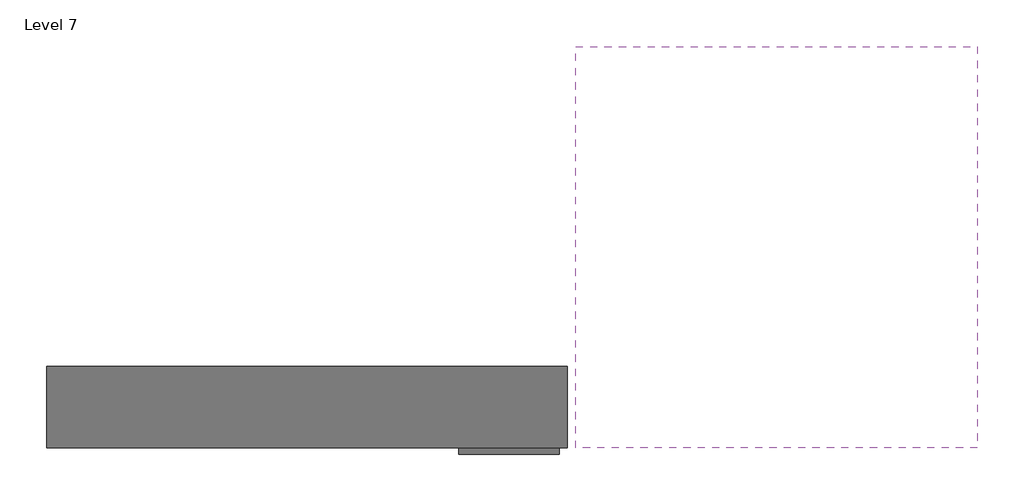
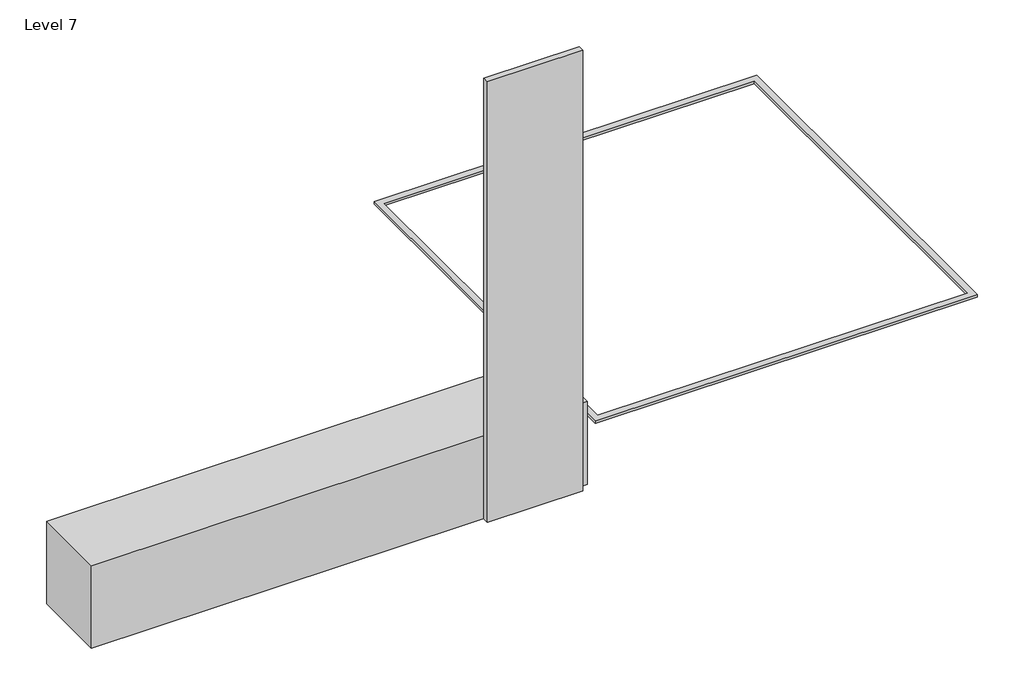
# One storey: 3 proxies.
"""IFC4 building model written with IfcOpenShell, lengths in millimetres."""

from ifc_helpers import new_model, si_unit, origin, place, context, project, spatial, transform, mapped, element, save
from components import generic_models_1_generic_models_1_aa688ddd, generic_models_6_generic_models_6_32940019, generic_models_7_generic_models_7_c575a30d

model = new_model("IFC4")

# Units and contexts
model_context = context("Model", 3, world=origin())
ifc_project = project(units=[si_unit("LENGTHUNIT", "METRE", prefix="MILLI")], contexts=[model_context])

# Site, building, storey
site = spatial("IfcSite", under=ifc_project)
building = spatial("IfcBuilding", under=site)
storey = spatial("IfcBuildingStorey", under=building, Name="Level 7", Elevation=1828.8)

# Proxies
placement = place(None, origin())
generic_models_1_generic_models_1_shape = generic_models_1_generic_models_1_aa688ddd(model_context)
element("IfcBuildingElementProxy", 1, Name="Generic Models 1 : Generic Models 1", ObjectType="Generic Models 1 : Generic Models 1", at=placement, inside=storey, context=model_context, shape_type="MappedRepresentation", body=[
    mapped(generic_models_1_generic_models_1_shape, transform((0.0, 0.0, 0.0), x_axis=(1.0, 0.0, 0.0), y_axis=(0.0, 1.0, 0.0), z_axis=(0.0, 0.0, 1.0))),
])
generic_models_6_generic_models_6_shape = generic_models_6_generic_models_6_32940019(model_context)
element("IfcBuildingElementProxy", 2, Name="Generic Models 6 : Generic Models 6", ObjectType="Generic Models 6 : Generic Models 6", at=placement, inside=storey, context=model_context, shape_type="MappedRepresentation", body=[
    mapped(generic_models_6_generic_models_6_shape, transform((0.0, 0.0, -660.4), x_axis=(1.0, 0.0, 0.0), y_axis=(0.0, 1.0, 0.0), z_axis=(0.0, 0.0, 1.0))),
])
generic_models_7_generic_models_7_shape = generic_models_7_generic_models_7_c575a30d(model_context)
element("IfcBuildingElementProxy", 3, Name="Generic Models 7 : Generic Models 7", ObjectType="Generic Models 7 : Generic Models 7", at=placement, inside=storey, context=model_context, shape_type="MappedRepresentation", body=[
    mapped(generic_models_7_generic_models_7_shape, transform((0.0, 0.0, 0.0), x_axis=(1.0, 0.0, 0.0), y_axis=(0.0, 1.0, 0.0), z_axis=(0.0, 0.0, 1.0))),
])

save(model, "model.ifc")

# Revit data of these elements
# Element 1 (IfcBuildingElementProxy, "Generic Models 1 : Generic Models 1")
#   Phase Created = New Construction
#   Materials on its faces: "Default New Material(1)"
# Element 2 (IfcBuildingElementProxy, "Generic Models 6 : Generic Models 6")
#   Phase Created = New Construction
# Element 3 (IfcBuildingElementProxy, "Generic Models 7 : Generic Models 7")
#   Phase Created = New Construction
#   Materials on its faces: "CLADDING WALL MATERIAL"
# Materials
#   "Default New Material(1)": class "Generic", colour RGB 120 120 120, transparency 0, Cost = 0
#   "CLADDING WALL MATERIAL": class "Generic", colour RGB 120 120 120, transparency 0, Cost = 0
